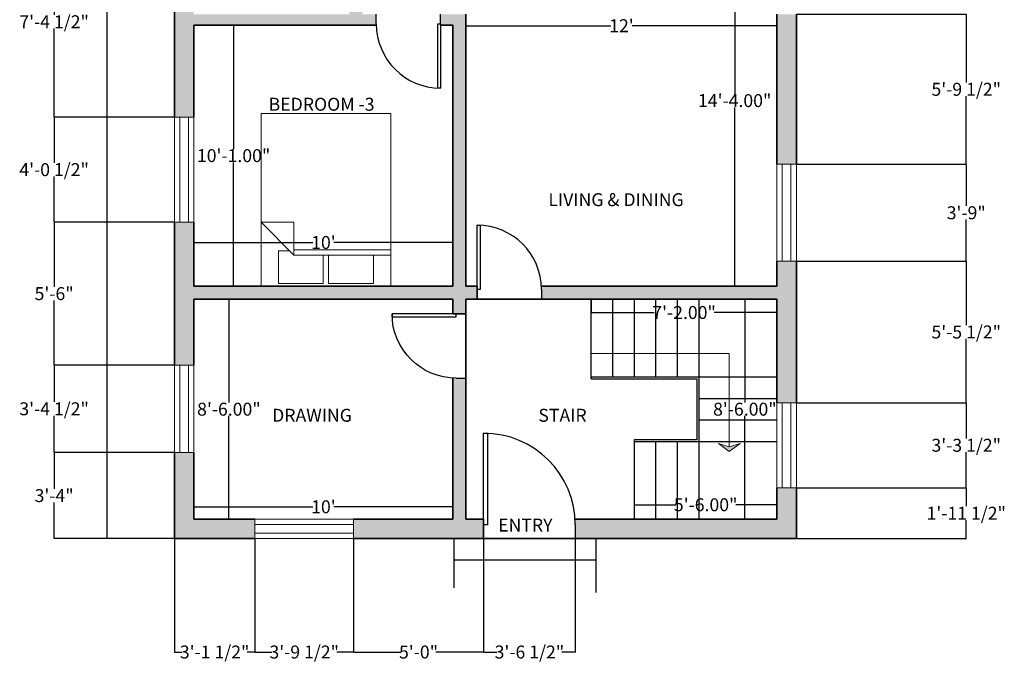
# Model space of a CAD drawing. Units: inches. Extents: x -54 to 402, y -41 to 548.
# Tile 1 of 2: x -54 to 402, y -41 to 261. Entities that reach past the tile are written whole.
import ezdxf

# ---------------------------------------------------------------- set-up
doc = ezdxf.new("R2010")
doc.units = ezdxf.units.IN
doc.header["$MEASUREMENT"] = 0
for name, color, linetype, lineweight in [('A-ANNO-DIMS', 2, 'Continuous', 18), ('A-ANNO-SYMB', 7, 'Continuous', 18), ('A-AREA-IDEN', 7, 'Continuous', 25), ('A-DOOR', 4, 'Continuous', 25), ('A-FLOR-STRS', 7, 'Continuous', 25), ('A-FURN', 8, 'Continuous', 18), ('A-GLAZ', 5, 'Continuous', 18), ('A-WALL', 7, 'Continuous', 35)]:
    doc.layers.add(name, color=color, linetype=linetype, lineweight=lineweight)
doc.layers.add('A-WALL-PATT', color=18, linetype='Continuous', lineweight=13, true_color=0x000000)
doc.styles.get("Standard").update_dxf_attribs({"font": 'arial.ttf'})
doc.dimstyles.get("Standard").update_dxf_attribs({"dimtxt": 6, "dimasz": 0.18, "dimexe": 0.18, "dimexo": 0.0625, "dimgap": 0.09, "dimtad": 0, "dimtih": 1, "dimtoh": 1, "dimzin": 0, "dimdsep": 46, "dimlunit": 3, "dimtxsty": 'Standard', "dimcen": 0.09, "dimadec": 0, "dimazin": 0, "dimtfac": 1, "dimtofl": 0, "dimtmove": 0, "dimatfit": 3, "dimfxl": 1, "dimtolj": 1, "dimtzin": 0, "dimarcsym": 0})

# ---------------------------------------------------------------- blocks, each defined once
blk = doc.blocks.new('*U2')
for p, q in [((0, 0), (0, -6)), ((40, 0), (40, -6))]:
    blk.add_line(p, q)
blk.add_lwpolyline([(0, 0), (0, 40), (1.75, 40), (1.75, 0)], close=True)
blk.add_arc((0, 0), 40, 0, 90)
blk = doc.blocks.new('Bed - Queen')
for p, q in [((0, -80.00003), (0, 0)), ((0, 0), (59.99999, 0)), ((59.99999, 0), (59.99999, -80.00003)), ((7.99999, -1.2), (28.79998, -1.2)), ((7.99999, -14.4), (7.99999, -1.2)), ((28.79998, -1.2), (28.79998, -14.4)), ((31.19999, -1.2), (51.99999, -1.2)), ((31.19999, -14.4), (31.19999, -1.2)), ((51.99999, -1.2), (51.99999, -16.4)), ((0, -14.4), (44.8, -14.4)), ((44.8, -16.8), (0, -16.8)), ((59.99999, -29.6), (44.8, -14.4)), ((44.8, -14.4), (44.8, -29.6)), ((51.99999, -16.4), (46.79936, -16.4)), ((44.8, -29.6), (59.99999, -29.6)), ((59.99999, -80.00003), (0, -80.00003))]:
    blk.add_line(p, q)
blk = doc.blocks.new('*D7')
at = {"layer": 'A-ANNO-DIMS', "color": 0, "lineweight": -2, "transparency": 16777216}
for p, q in [((18.01, 524.86), (-13.3, 524.86)), ((-13.12, 524.68), (-13.12, 275.96)), ((-13.12, 21.04), (-13.12, 269.76)), ((18.01, 20.86), (-13.3, 20.86))]:
    blk.add_line(p, q, dxfattribs=at)
at = {"layer": 'A-ANNO-DIMS', "color": 0, "transparency": 16777216}
for points in [[(-13.15, 524.68), (-13.09, 524.68), (-13.12, 524.86)], [(-13.15, 21.04), (-13.09, 21.04), (-13.12, 20.86)]]:
    blk.add_solid(points, dxfattribs=at)
at = {"layer": 'Defpoints', "color": 0, "transparency": 16777216}
for p in [(18.08, 524.86), (-13.12, 20.86), (18.08, 20.86)]:
    blk.add_point(p, dxfattribs=at)
at = {"layer": 'A-ANNO-DIMS', "color": 0, "transparency": 16777216, "insert": (-13.12, 272.86), "char_height": 6, "attachment_point": 5}
blk.add_mtext("\\A1;42'", dxfattribs=at)
blk = doc.blocks.new('*D8')
at = {"layer": 'A-ANNO-DIMS', "color": 0, "lineweight": -2, "transparency": 16777216}
for p, q in [((211.08, 131.8), (211.08, 125.48)), ((297.08, 131.8), (297.08, 125.48)), ((211.26, 125.66), (240.21, 125.66)), ((296.9, 125.66), (267.94, 125.66))]:
    blk.add_line(p, q, dxfattribs=at)
at = {"layer": 'A-ANNO-DIMS', "color": 0, "transparency": 16777216}
for points in [[(211.26, 125.69), (211.26, 125.63), (211.08, 125.66)], [(296.9, 125.69), (296.9, 125.63), (297.08, 125.66)]]:
    blk.add_solid(points, dxfattribs=at)
at = {"layer": 'Defpoints', "color": 0, "transparency": 16777216}
for p in [(211.08, 131.86), (297.08, 131.86), (297.08, 125.66)]:
    blk.add_point(p, dxfattribs=at)
at = {"layer": 'A-ANNO-DIMS', "color": 0, "transparency": 16777216, "insert": (254.08, 125.66), "char_height": 6, "attachment_point": 5}
blk.add_mtext('\\A1;7\'-2.00"', dxfattribs=at)
blk = doc.blocks.new('*D9')
at = {"layer": 'A-ANNO-DIMS', "color": 0, "lineweight": -2, "transparency": 16777216}
for p, q in [((231.08, 29.92), (231.08, 36.75)), ((231.26, 36.57), (250.19, 36.57)), ((296.9, 36.57), (277.97, 36.57)), ((297.08, 29.92), (297.08, 36.75))]:
    blk.add_line(p, q, dxfattribs=at)
at = {"layer": 'A-ANNO-DIMS', "color": 0, "transparency": 16777216}
for points in [[(231.26, 36.6), (231.26, 36.54), (231.08, 36.57)], [(296.9, 36.6), (296.9, 36.54), (297.08, 36.57)]]:
    blk.add_solid(points, dxfattribs=at)
at = {"layer": 'Defpoints', "color": 0, "transparency": 16777216}
for p in [(297.08, 36.57), (231.08, 29.86), (297.08, 29.86)]:
    blk.add_point(p, dxfattribs=at)
at = {"layer": 'A-ANNO-DIMS', "color": 0, "transparency": 16777216, "insert": (264.08, 36.57), "char_height": 6, "attachment_point": 5}
blk.add_mtext('\\A1;5\'-6.00"', dxfattribs=at)
blk = doc.blocks.new('*D10')
at = {"layer": 'A-ANNO-DIMS', "color": 0, "lineweight": -2, "transparency": 16777216}
for p, q in [((297.01, 131.86), (282.05, 131.86)), ((282.23, 131.68), (282.23, 84.01)), ((282.23, 30.04), (282.23, 77.71)), ((297.01, 29.86), (282.05, 29.86))]:
    blk.add_line(p, q, dxfattribs=at)
at = {"layer": 'A-ANNO-DIMS', "color": 0, "transparency": 16777216}
for points in [[(282.2, 131.68), (282.26, 131.68), (282.23, 131.86)], [(282.2, 30.04), (282.26, 30.04), (282.23, 29.86)]]:
    blk.add_solid(points, dxfattribs=at)
at = {"layer": 'Defpoints', "color": 0, "transparency": 16777216}
for p in [(297.08, 131.86), (282.23, 29.86), (297.08, 29.86)]:
    blk.add_point(p, dxfattribs=at)
at = {"layer": 'A-ANNO-DIMS', "color": 0, "transparency": 16777216, "insert": (282.23, 80.86), "char_height": 6, "attachment_point": 5}
blk.add_mtext('\\A1;8\'-6.00"', dxfattribs=at)
blk = doc.blocks.new('*D11')
at = {"layer": 'A-ANNO-DIMS', "color": 0, "lineweight": -2, "transparency": 16777216}
for p, q in [((27.08, 29.92), (27.08, 35.81)), ((27.26, 35.63), (82.18, 35.63)), ((146.9, 35.63), (91.98, 35.63)), ((147.08, 29.92), (147.08, 35.81))]:
    blk.add_line(p, q, dxfattribs=at)
at = {"layer": 'A-ANNO-DIMS', "color": 0, "transparency": 16777216}
for points in [[(27.26, 35.66), (27.26, 35.6), (27.08, 35.63)], [(146.9, 35.66), (146.9, 35.6), (147.08, 35.63)]]:
    blk.add_solid(points, dxfattribs=at)
at = {"layer": 'Defpoints', "color": 0, "transparency": 16777216}
for p in [(147.08, 35.63), (27.08, 29.86), (147.08, 29.86)]:
    blk.add_point(p, dxfattribs=at)
at = {"layer": 'A-ANNO-DIMS', "color": 0, "transparency": 16777216, "insert": (87.08, 35.63), "char_height": 6, "attachment_point": 5}
blk.add_mtext("\\A1;10'", dxfattribs=at)
blk = doc.blocks.new('*D12')
at = {"layer": 'A-ANNO-DIMS', "color": 0, "lineweight": -2, "transparency": 16777216}
for p, q in [((27.14, 131.86), (43.5, 131.86)), ((43.32, 131.68), (43.32, 84.01)), ((43.32, 30.04), (43.32, 77.71)), ((27.14, 29.86), (43.5, 29.86))]:
    blk.add_line(p, q, dxfattribs=at)
at = {"layer": 'A-ANNO-DIMS', "color": 0, "transparency": 16777216}
for points in [[(43.29, 131.68), (43.35, 131.68), (43.32, 131.86)], [(43.29, 30.04), (43.35, 30.04), (43.32, 29.86)]]:
    blk.add_solid(points, dxfattribs=at)
at = {"layer": 'Defpoints', "color": 0, "transparency": 16777216}
for p in [(27.08, 131.86), (27.08, 29.86), (43.32, 29.86)]:
    blk.add_point(p, dxfattribs=at)
at = {"layer": 'A-ANNO-DIMS', "color": 0, "transparency": 16777216, "insert": (43.32, 80.86), "char_height": 6, "attachment_point": 5}
blk.add_mtext('\\A1;8\'-6.00"', dxfattribs=at)
blk = doc.blocks.new('*D13')
at = {"layer": 'A-ANNO-DIMS', "color": 0, "lineweight": -2, "transparency": 16777216}
for p, q in [((27.08, 137.92), (27.08, 158.29)), ((27.26, 158.11), (82.18, 158.11)), ((146.9, 158.11), (91.98, 158.11)), ((147.08, 137.92), (147.08, 158.29))]:
    blk.add_line(p, q, dxfattribs=at)
at = {"layer": 'A-ANNO-DIMS', "color": 0, "transparency": 16777216}
for points in [[(27.26, 158.14), (27.26, 158.08), (27.08, 158.11)], [(146.9, 158.14), (146.9, 158.08), (147.08, 158.11)]]:
    blk.add_solid(points, dxfattribs=at)
at = {"layer": 'Defpoints', "color": 0, "transparency": 16777216}
for p in [(147.08, 158.11), (27.08, 137.86), (147.08, 137.86)]:
    blk.add_point(p, dxfattribs=at)
at = {"layer": 'A-ANNO-DIMS', "color": 0, "transparency": 16777216, "insert": (87.08, 158.11), "char_height": 6, "attachment_point": 5}
blk.add_mtext("\\A1;10'", dxfattribs=at)
blk = doc.blocks.new('*D14')
at = {"layer": 'A-ANNO-DIMS', "color": 0, "lineweight": -2, "transparency": 16777216}
for p, q in [((27.14, 258.86), (45.68, 258.86)), ((45.5, 258.68), (45.5, 201.51)), ((45.5, 138.04), (45.5, 195.21)), ((27.14, 137.86), (45.68, 137.86))]:
    blk.add_line(p, q, dxfattribs=at)
at = {"layer": 'A-ANNO-DIMS', "color": 0, "transparency": 16777216}
for points in [[(45.47, 258.68), (45.53, 258.68), (45.5, 258.86)], [(45.47, 138.04), (45.53, 138.04), (45.5, 137.86)]]:
    blk.add_solid(points, dxfattribs=at)
at = {"layer": 'Defpoints', "color": 0, "transparency": 16777216}
for p in [(27.08, 258.86), (27.08, 137.86), (45.5, 137.86)]:
    blk.add_point(p, dxfattribs=at)
at = {"layer": 'A-ANNO-DIMS', "color": 0, "transparency": 16777216, "insert": (45.5, 198.36), "char_height": 6, "attachment_point": 5}
blk.add_mtext('\\A1;10\'-1.00"', dxfattribs=at)
blk = doc.blocks.new('*D15')
at = {"layer": 'A-ANNO-DIMS', "color": 0, "lineweight": -2, "transparency": 16777216}
for p, q in [((153.08, 263.8), (153.08, 258.38)), ((297.08, 263.8), (297.08, 258.38)), ((153.26, 258.56), (220.18, 258.56)), ((296.9, 258.56), (229.98, 258.56))]:
    blk.add_line(p, q, dxfattribs=at)
at = {"layer": 'A-ANNO-DIMS', "color": 0, "transparency": 16777216}
for points in [[(153.26, 258.59), (153.26, 258.53), (153.08, 258.56)], [(296.9, 258.59), (296.9, 258.53), (297.08, 258.56)]]:
    blk.add_solid(points, dxfattribs=at)
at = {"layer": 'Defpoints', "color": 0, "transparency": 16777216}
for p in [(153.08, 263.86), (297.08, 263.86), (297.08, 258.56)]:
    blk.add_point(p, dxfattribs=at)
at = {"layer": 'A-ANNO-DIMS', "color": 0, "transparency": 16777216, "insert": (225.08, 258.56), "char_height": 6, "attachment_point": 5}
blk.add_mtext("\\A1;12'", dxfattribs=at)
blk = doc.blocks.new('*D16')
at = {"layer": 'A-ANNO-DIMS', "color": 0, "lineweight": -2, "transparency": 16777216}
for p, q in [((297.01, 309.86), (277.33, 309.86)), ((277.51, 309.68), (277.51, 227.01)), ((277.51, 138.04), (277.51, 220.71)), ((297.01, 137.86), (277.33, 137.86))]:
    blk.add_line(p, q, dxfattribs=at)
at = {"layer": 'A-ANNO-DIMS', "color": 0, "transparency": 16777216}
for points in [[(277.48, 309.68), (277.54, 309.68), (277.51, 309.86)], [(277.48, 138.04), (277.54, 138.04), (277.51, 137.86)]]:
    blk.add_solid(points, dxfattribs=at)
at = {"layer": 'Defpoints', "color": 0, "transparency": 16777216}
for p in [(297.08, 309.86), (277.51, 137.86), (297.08, 137.86)]:
    blk.add_point(p, dxfattribs=at)
at = {"layer": 'A-ANNO-DIMS', "color": 0, "transparency": 16777216, "insert": (277.51, 223.86), "char_height": 6, "attachment_point": 5}
blk.add_mtext('\\A1;14\'-4.00"', dxfattribs=at)
blk = doc.blocks.new('*D32')
at = {"layer": 'A-ANNO-DIMS', "color": 0, "lineweight": -2, "transparency": 16777216}
for p, q in [((18.01, 60.78), (-37.79, 60.78)), ((-37.61, 60.6), (-37.61, 43.98)), ((-37.61, 21.04), (-37.61, 37.67)), ((18.01, 20.86), (-37.79, 20.86))]:
    blk.add_line(p, q, dxfattribs=at)
at = {"layer": 'A-ANNO-DIMS', "color": 0, "transparency": 16777216}
for points in [[(-37.64, 60.6), (-37.58, 60.6), (-37.61, 60.78)], [(-37.64, 21.04), (-37.58, 21.04), (-37.61, 20.86)]]:
    blk.add_solid(points, dxfattribs=at)
at = {"layer": 'Defpoints', "color": 0, "transparency": 16777216}
for p in [(-37.61, 60.78), (18.08, 60.78), (18.08, 20.86)]:
    blk.add_point(p, dxfattribs=at)
at = {"layer": 'A-ANNO-DIMS', "color": 0, "transparency": 16777216, "insert": (-37.61, 40.82), "char_height": 6, "attachment_point": 5}
blk.add_mtext('\\A1;3\'-4"', dxfattribs=at)
blk = doc.blocks.new('*D33')
at = {"layer": 'A-ANNO-DIMS', "color": 0, "lineweight": -2, "transparency": 16777216}
for p, q in [((18.01, 101.29), (-37.79, 101.29)), ((-37.61, 101.11), (-37.61, 84.23)), ((-37.61, 60.96), (-37.61, 77.84)), ((18.01, 60.78), (-37.79, 60.78))]:
    blk.add_line(p, q, dxfattribs=at)
at = {"layer": 'A-ANNO-DIMS', "color": 0, "transparency": 16777216}
for points in [[(-37.64, 101.11), (-37.58, 101.11), (-37.61, 101.29)], [(-37.64, 60.96), (-37.58, 60.96), (-37.61, 60.78)]]:
    blk.add_solid(points, dxfattribs=at)
at = {"layer": 'Defpoints', "color": 0, "transparency": 16777216}
for p in [(-37.61, 101.29), (18.08, 101.29), (18.08, 60.78)]:
    blk.add_point(p, dxfattribs=at)
at = {"layer": 'A-ANNO-DIMS', "color": 0, "transparency": 16777216, "insert": (-37.61, 81.04), "char_height": 6, "attachment_point": 5}
blk.add_mtext('\\A1;3\'-4 1/2"', dxfattribs=at)
blk = doc.blocks.new('*D34')
at = {"layer": 'A-ANNO-DIMS', "color": 0, "lineweight": -2, "transparency": 16777216}
for p, q in [((18.01, 167.53), (-37.79, 167.53)), ((-37.61, 167.35), (-37.61, 137.56)), ((-37.61, 101.47), (-37.61, 131.26)), ((18.01, 101.29), (-37.79, 101.29))]:
    blk.add_line(p, q, dxfattribs=at)
at = {"layer": 'A-ANNO-DIMS', "color": 0, "transparency": 16777216}
for points in [[(-37.64, 167.35), (-37.58, 167.35), (-37.61, 167.53)], [(-37.64, 101.47), (-37.58, 101.47), (-37.61, 101.29)]]:
    blk.add_solid(points, dxfattribs=at)
at = {"layer": 'Defpoints', "color": 0, "transparency": 16777216}
for p in [(-37.61, 167.53), (18.08, 167.53), (18.08, 101.29)]:
    blk.add_point(p, dxfattribs=at)
at = {"layer": 'A-ANNO-DIMS', "color": 0, "transparency": 16777216, "insert": (-37.61, 134.41), "char_height": 6, "attachment_point": 5}
blk.add_mtext('\\A1;5\'-6"', dxfattribs=at)
blk = doc.blocks.new('*D35')
at = {"layer": 'A-ANNO-DIMS', "color": 0, "lineweight": -2, "transparency": 16777216}
for p, q in [((18.01, 216.22), (-37.79, 216.22)), ((-37.61, 216.04), (-37.61, 195.07)), ((-37.61, 167.71), (-37.61, 188.68)), ((18.01, 167.53), (-37.79, 167.53))]:
    blk.add_line(p, q, dxfattribs=at)
at = {"layer": 'A-ANNO-DIMS', "color": 0, "transparency": 16777216}
for points in [[(-37.64, 216.04), (-37.58, 216.04), (-37.61, 216.22)], [(-37.64, 167.71), (-37.58, 167.71), (-37.61, 167.53)]]:
    blk.add_solid(points, dxfattribs=at)
at = {"layer": 'Defpoints', "color": 0, "transparency": 16777216}
for p in [(-37.61, 216.22), (18.08, 216.22), (18.08, 167.53)]:
    blk.add_point(p, dxfattribs=at)
at = {"layer": 'A-ANNO-DIMS', "color": 0, "transparency": 16777216, "insert": (-37.61, 191.87), "char_height": 6, "attachment_point": 5}
blk.add_mtext('\\A1;4\'-0 1/2"', dxfattribs=at)
blk = doc.blocks.new('*D36')
at = {"layer": 'A-ANNO-DIMS', "color": 0, "lineweight": -2, "transparency": 16777216}
for p, q in [((18.01, 304.58), (-37.79, 304.58)), ((-37.61, 304.4), (-37.61, 263.59)), ((-37.61, 216.4), (-37.61, 257.21)), ((18.01, 216.22), (-37.79, 216.22))]:
    blk.add_line(p, q, dxfattribs=at)
at = {"layer": 'A-ANNO-DIMS', "color": 0, "transparency": 16777216}
for points in [[(-37.64, 304.4), (-37.58, 304.4), (-37.61, 304.58)], [(-37.64, 216.4), (-37.58, 216.4), (-37.61, 216.22)]]:
    blk.add_solid(points, dxfattribs=at)
at = {"layer": 'Defpoints', "color": 0, "transparency": 16777216}
for p in [(-37.61, 304.58), (18.08, 304.58), (18.08, 216.22)]:
    blk.add_point(p, dxfattribs=at)
at = {"layer": 'A-ANNO-DIMS', "color": 0, "transparency": 16777216, "insert": (-37.61, 260.4), "char_height": 6, "attachment_point": 5}
blk.add_mtext('\\A1;7\'-4 1/2"', dxfattribs=at)
blk = doc.blocks.new('*D39')
at = {"layer": 'A-ANNO-DIMS', "color": 0, "lineweight": -2, "transparency": 16777216}
for p, q in [((306.14, 44.45), (384.91, 44.45)), ((384.73, 44.27), (384.73, 35.85)), ((384.73, 21.04), (384.73, 29.46)), ((306.14, 20.86), (384.91, 20.86))]:
    blk.add_line(p, q, dxfattribs=at)
at = {"layer": 'A-ANNO-DIMS', "color": 0, "transparency": 16777216}
for points in [[(384.7, 44.27), (384.76, 44.27), (384.73, 44.45)], [(384.7, 21.04), (384.76, 21.04), (384.73, 20.86)]]:
    blk.add_solid(points, dxfattribs=at)
at = {"layer": 'Defpoints', "color": 0, "transparency": 16777216}
for p in [(306.08, 44.45), (384.73, 44.45), (306.08, 20.86)]:
    blk.add_point(p, dxfattribs=at)
at = {"layer": 'A-ANNO-DIMS', "color": 0, "transparency": 16777216, "insert": (384.73, 32.65), "char_height": 6, "attachment_point": 5}
blk.add_mtext('\\A1;1\'-11 1/2"', dxfattribs=at)
blk = doc.blocks.new('*D40')
at = {"layer": 'A-ANNO-DIMS', "color": 0, "lineweight": -2, "transparency": 16777216}
for p, q in [((306.14, 83.84), (384.91, 83.84)), ((384.73, 83.66), (384.73, 67.34)), ((384.73, 44.63), (384.73, 60.95)), ((306.14, 44.45), (384.91, 44.45))]:
    blk.add_line(p, q, dxfattribs=at)
at = {"layer": 'A-ANNO-DIMS', "color": 0, "transparency": 16777216}
for points in [[(384.7, 83.66), (384.76, 83.66), (384.73, 83.84)], [(384.7, 44.63), (384.76, 44.63), (384.73, 44.45)]]:
    blk.add_solid(points, dxfattribs=at)
at = {"layer": 'Defpoints', "color": 0, "transparency": 16777216}
for p in [(306.08, 83.84), (384.73, 83.84), (306.08, 44.45)]:
    blk.add_point(p, dxfattribs=at)
at = {"layer": 'A-ANNO-DIMS', "color": 0, "transparency": 16777216, "insert": (384.73, 64.14), "char_height": 6, "attachment_point": 5}
blk.add_mtext('\\A1;3\'-3 1/2"', dxfattribs=at)
blk = doc.blocks.new('*D41')
at = {"layer": 'A-ANNO-DIMS', "color": 0, "lineweight": -2, "transparency": 16777216}
for p, q in [((306.14, 149.43), (384.91, 149.43)), ((384.73, 149.25), (384.73, 119.83)), ((384.73, 84.02), (384.73, 113.44)), ((306.14, 83.84), (384.91, 83.84))]:
    blk.add_line(p, q, dxfattribs=at)
at = {"layer": 'A-ANNO-DIMS', "color": 0, "transparency": 16777216}
for points in [[(384.7, 149.25), (384.76, 149.25), (384.73, 149.43)], [(384.7, 84.02), (384.76, 84.02), (384.73, 83.84)]]:
    blk.add_solid(points, dxfattribs=at)
at = {"layer": 'Defpoints', "color": 0, "transparency": 16777216}
for p in [(306.08, 149.43), (384.73, 149.43), (306.08, 83.84)]:
    blk.add_point(p, dxfattribs=at)
at = {"layer": 'A-ANNO-DIMS', "color": 0, "transparency": 16777216, "insert": (384.73, 116.63), "char_height": 6, "attachment_point": 5}
blk.add_mtext('\\A1;5\'-5 1/2"', dxfattribs=at)
blk = doc.blocks.new('*D42')
at = {"layer": 'A-ANNO-DIMS', "color": 0, "lineweight": -2, "transparency": 16777216}
for p, q in [((306.14, 194.33), (384.91, 194.33)), ((384.73, 194.15), (384.73, 175.04)), ((384.73, 149.61), (384.73, 168.73)), ((306.14, 149.43), (384.91, 149.43))]:
    blk.add_line(p, q, dxfattribs=at)
at = {"layer": 'A-ANNO-DIMS', "color": 0, "transparency": 16777216}
for points in [[(384.7, 194.15), (384.76, 194.15), (384.73, 194.33)], [(384.7, 149.61), (384.76, 149.61), (384.73, 149.43)]]:
    blk.add_solid(points, dxfattribs=at)
at = {"layer": 'Defpoints', "color": 0, "transparency": 16777216}
for p in [(306.08, 194.33), (384.73, 194.33), (306.08, 149.43)]:
    blk.add_point(p, dxfattribs=at)
at = {"layer": 'A-ANNO-DIMS', "color": 0, "transparency": 16777216, "insert": (384.73, 171.88), "char_height": 6, "attachment_point": 5}
blk.add_mtext('\\A1;3\'-9"', dxfattribs=at)
blk = doc.blocks.new('*D43')
at = {"layer": 'A-ANNO-DIMS', "color": 0, "lineweight": -2, "transparency": 16777216}
for p, q in [((306.14, 263.86), (384.91, 263.86)), ((384.73, 263.68), (384.73, 232.29)), ((384.73, 194.51), (384.73, 225.91)), ((306.14, 194.33), (384.91, 194.33))]:
    blk.add_line(p, q, dxfattribs=at)
at = {"layer": 'A-ANNO-DIMS', "color": 0, "transparency": 16777216}
for points in [[(384.7, 263.68), (384.76, 263.68), (384.73, 263.86)], [(384.7, 194.51), (384.76, 194.51), (384.73, 194.33)]]:
    blk.add_solid(points, dxfattribs=at)
at = {"layer": 'Defpoints', "color": 0, "transparency": 16777216}
for p in [(306.08, 263.86), (384.73, 263.86), (306.08, 194.33)]:
    blk.add_point(p, dxfattribs=at)
at = {"layer": 'A-ANNO-DIMS', "color": 0, "transparency": 16777216, "insert": (384.73, 229.1), "char_height": 6, "attachment_point": 5}
blk.add_mtext('\\A1;5\'-9 1/2"', dxfattribs=at)
blk = doc.blocks.new('*D48')
at = {"layer": 'A-ANNO-DIMS', "color": 0, "lineweight": -2, "transparency": 16777216}
for p, q in [((18.08, 20.8), (18.08, -31.85)), ((55.33, 20.8), (55.33, -31.85)), ((18.26, -31.67), (21.65, -31.67)), ((55.15, -31.67), (51.76, -31.67))]:
    blk.add_line(p, q, dxfattribs=at)
at = {"layer": 'A-ANNO-DIMS', "color": 0, "transparency": 16777216}
for points in [[(18.26, -31.64), (18.26, -31.7), (18.08, -31.67)], [(55.15, -31.64), (55.15, -31.7), (55.33, -31.67)]]:
    blk.add_solid(points, dxfattribs=at)
at = {"layer": 'Defpoints', "color": 0, "transparency": 16777216}
for p in [(18.08, 20.86), (55.33, 20.86), (55.33, -31.67)]:
    blk.add_point(p, dxfattribs=at)
at = {"layer": 'A-ANNO-DIMS', "color": 0, "transparency": 16777216, "insert": (36.71, -31.67), "char_height": 6, "attachment_point": 5}
blk.add_mtext('\\A1;3\'-1 1/2"', dxfattribs=at)
blk = doc.blocks.new('*D49')
at = {"layer": 'A-ANNO-DIMS', "color": 0, "lineweight": -2, "transparency": 16777216}
for p, q in [((55.33, 20.8), (55.33, -31.85)), ((101.04, 20.8), (101.04, -31.85)), ((55.51, -31.67), (63.13, -31.67)), ((100.86, -31.67), (93.24, -31.67))]:
    blk.add_line(p, q, dxfattribs=at)
at = {"layer": 'A-ANNO-DIMS', "color": 0, "transparency": 16777216}
for points in [[(55.51, -31.64), (55.51, -31.7), (55.33, -31.67)], [(100.86, -31.64), (100.86, -31.7), (101.04, -31.67)]]:
    blk.add_solid(points, dxfattribs=at)
at = {"layer": 'Defpoints', "color": 0, "transparency": 16777216}
for p in [(55.33, 20.86), (101.04, 20.86), (101.04, -31.67)]:
    blk.add_point(p, dxfattribs=at)
at = {"layer": 'A-ANNO-DIMS', "color": 0, "transparency": 16777216, "insert": (78.19, -31.67), "char_height": 6, "attachment_point": 5}
blk.add_mtext('\\A1;3\'-9 1/2"', dxfattribs=at)
blk = doc.blocks.new('*D50')
at = {"layer": 'A-ANNO-DIMS', "color": 0, "lineweight": -2, "transparency": 16777216}
for p, q in [((101.04, 20.8), (101.04, -31.85)), ((161.22, 20.8), (161.22, -31.85)), ((101.22, -31.67), (123.07, -31.67)), ((161.04, -31.67), (139.2, -31.67))]:
    blk.add_line(p, q, dxfattribs=at)
at = {"layer": 'A-ANNO-DIMS', "color": 0, "transparency": 16777216}
for points in [[(101.22, -31.64), (101.22, -31.7), (101.04, -31.67)], [(161.04, -31.64), (161.04, -31.7), (161.22, -31.67)]]:
    blk.add_solid(points, dxfattribs=at)
at = {"layer": 'Defpoints', "color": 0, "transparency": 16777216}
for p in [(101.04, 20.86), (161.22, 20.86), (161.22, -31.67)]:
    blk.add_point(p, dxfattribs=at)
at = {"layer": 'A-ANNO-DIMS', "color": 0, "transparency": 16777216, "insert": (131.13, -31.67), "char_height": 6, "attachment_point": 5}
blk.add_mtext('\\A1;5\'-0"', dxfattribs=at)
blk = doc.blocks.new('*D51')
at = {"layer": 'A-ANNO-DIMS', "color": 0, "lineweight": -2, "transparency": 16777216}
for p, q in [((161.22, 20.8), (161.22, -31.85)), ((203.72, 20.8), (203.72, -31.85)), ((161.4, -31.67), (167.42, -31.67)), ((203.54, -31.67), (197.53, -31.67))]:
    blk.add_line(p, q, dxfattribs=at)
at = {"layer": 'A-ANNO-DIMS', "color": 0, "transparency": 16777216}
for points in [[(161.4, -31.64), (161.4, -31.7), (161.22, -31.67)], [(203.54, -31.64), (203.54, -31.7), (203.72, -31.67)]]:
    blk.add_solid(points, dxfattribs=at)
at = {"layer": 'Defpoints', "color": 0, "transparency": 16777216}
for p in [(161.22, 20.86), (203.72, 20.86), (203.72, -31.67)]:
    blk.add_point(p, dxfattribs=at)
at = {"layer": 'A-ANNO-DIMS', "color": 0, "transparency": 16777216, "insert": (182.47, -31.67), "char_height": 6, "attachment_point": 5}
blk.add_mtext('\\A1;3\'-6 1/2"', dxfattribs=at)

msp = doc.modelspace()

# ---------------------------------------------------------------- hatches: boundary and pattern name
at = {"layer": 'A-ANNO-SYMB'}
h = msp.add_hatch(color=256, dxfattribs=at)
h.dxf.hatch_style = 1
h.paths.add_polyline_path([(280.116, 65.005), (274.889, 63.445), (269.955, 65.034), (274.889, 61.274)])
at = {"layer": 'A-WALL-PATT'}
h = msp.add_hatch(color=256, dxfattribs=at)
h.dxf.hatch_style = 1
h.paths.add_polyline_path([(306.077, 149.429), (297.077, 149.429), (297.077, 137.861), (188.036, 137.861, -0.0129064), (188.075, 136.326), (188.075, 131.861), (297.077, 131.861), (297.077, 83.839), (306.077, 83.839)])
h.paths.add_polyline_path([(306.077, 263.861), (297.077, 263.861), (297.077, 194.333), (306.077, 194.333)])
h.paths.add_polyline_path([(306.077, 44.446), (297.077, 44.446), (297.077, 29.861), (203.639, 29.861, -0.015458), (203.72, 27.236), (203.72, 20.861), (306.077, 20.861)])
h.paths.add_polyline_path([(55.334, 29.861), (27.077, 29.861), (27.077, 60.781), (18.077, 60.781), (18.077, 20.861), (55.334, 20.861)])
h.paths.add_polyline_path([(161.225, 27.236), (161.225, 29.861), (153.077, 29.861), (153.077, 95.263), (148.613, 95.263, -0.0129064), (147.077, 95.303), (147.077, 29.861), (101.039, 29.861), (101.039, 20.861), (161.225, 20.861)])
h.paths.add_polyline_path([(158.313, 136.326), (158.313, 137.861), (153.077, 137.861), (153.077, 263.861), (141.33, 263.861), (141.33, 259.397), (141.33, 258.861), (147.077, 258.861), (147.077, 137.861), (27.077, 137.861), (27.077, 167.529), (18.077, 167.529), (18.077, 101.294), (27.077, 101.294), (27.077, 131.861), (147.077, 131.861), (147.077, 125.025), (148.613, 125.025), (153.077, 125.025), (153.077, 131.861), (158.313, 131.861)])
h.paths.add_polyline_path([(111.568, 263.861), (105.077, 263.861), (105.077, 293.745), (99.077, 293.745), (99.077, 263.861), (27.077, 263.861), (27.077, 304.579), (18.077, 304.579), (18.077, 216.221), (27.077, 216.221), (27.077, 258.861), (111.573, 258.861, -0.0045002), (111.568, 259.397)])
h.paths.add_polyline_path([(112.102, 364.326, -0.0129064), (112.142, 365.861), (27.077, 365.861), (27.077, 402.028), (18.077, 402.028), (18.077, 335.061), (27.077, 335.061), (27.077, 359.861), (99.077, 359.861), (99.077, 331.859), (105.077, 331.859), (105.077, 359.861), (112.102, 359.861)])

# ---------------------------------------------------------------- linework, layer by layer
at = {"layer": 'A-ANNO-SYMB'}
for p, q in [((211.077, 106.597), (274.889, 106.597)), ((274.889, 106.597), (274.889, 63.445)), ((274.889, 61.274), (269.955, 65.034)), ((274.889, 63.445), (269.955, 65.034)), ((274.889, 61.274), (280.116, 65.005)), ((280.116, 65.005), (274.889, 61.274)), ((274.889, 63.445), (280.116, 65.005))]:
    msp.add_line(p, q, dxfattribs=at)
at = {"layer": 'A-DOOR'}
msp.add_lwpolyline([(161.225, 27.361), (163.084, 27.361)], dxfattribs=at)
at = {"layer": 'A-FLOR-STRS'}
for p, q in [((261.077, 95.861), (297.077, 95.861)), ((261.077, 85.861), (297.077, 85.861)), ((261.077, 75.861), (297.077, 75.861)), ((261.077, 65.861), (297.077, 65.861)), ((147.465, 20.861), (147.465, -1.916)), ((213.19, 20.861), (213.19, -4.018)), ((147.465, 11.118), (213.19, 11.118))]:
    msp.add_line(p, q, dxfattribs=at)
for points in [[(211.077, 94.861), (211.077, 131.861)], [(221.077, 95.861), (221.077, 131.861)], [(231.077, 95.861), (231.077, 131.861)], [(241.077, 95.861), (241.077, 131.861)], [(251.077, 95.861), (251.077, 131.861)], [(261.077, 29.861), (261.077, 131.861)], [(211.077, 95.861), (261.077, 95.861)], [(211.077, 94.861), (260.077, 94.861)], [(260.077, 66.861), (260.077, 94.861)], [(231.077, 29.861), (231.077, 66.861)], [(231.077, 66.861), (260.077, 66.861)], [(231.077, 65.861), (261.077, 65.861)], [(241.077, 29.861), (241.077, 65.861)], [(251.077, 29.861), (251.077, 65.861)]]:
    msp.add_lwpolyline(points, dxfattribs=at)
at = {"layer": 'A-GLAZ'}
for p, q in [((27.077, 216.221), (18.077, 216.221)), ((297.077, 194.333), (306.077, 194.333)), ((27.077, 167.529), (18.077, 167.529)), ((297.077, 149.429), (306.077, 149.429)), ((27.077, 101.294), (18.077, 101.294)), ((297.077, 83.839), (306.077, 83.839)), ((27.077, 60.781), (18.077, 60.781)), ((297.077, 44.446), (306.077, 44.446)), ((55.334, 29.861), (55.334, 20.861)), ((101.039, 29.861), (101.039, 20.861))]:
    msp.add_line(p, q, dxfattribs=at)
for points in [[(18.077, 216.221), (27.077, 216.221), (27.077, 167.529), (18.077, 167.529)], [(297.077, 194.333), (306.077, 194.333), (306.077, 149.429), (297.077, 149.429)], [(18.077, 101.294), (27.077, 101.294), (27.077, 60.781), (18.077, 60.781)], [(297.077, 83.839), (306.077, 83.839), (306.077, 44.446), (297.077, 44.446)], [(55.334, 29.861), (101.039, 29.861), (101.039, 20.861), (55.334, 20.861)]]:
    msp.add_lwpolyline(points, close=True, dxfattribs=at)
for points in [[(20.577, 216.221), (20.577, 167.529)], [(24.577, 216.221), (24.577, 167.529)], [(299.577, 149.429), (299.577, 194.333)], [(303.577, 149.429), (303.577, 194.333)], [(20.577, 101.294), (20.577, 60.781)], [(24.577, 101.294), (24.577, 60.781)], [(299.577, 44.446), (299.577, 83.839)], [(303.577, 44.446), (303.577, 83.839)], [(55.334, 27.361), (101.039, 27.361)], [(55.334, 23.361), (101.039, 23.361)]]:
    msp.add_lwpolyline(points, dxfattribs=at)
at = {"layer": 'A-WALL'}
for p, q in [((297.077, 137.861), (297.077, 149.429)), ((158.313, 137.861), (158.313, 131.861)), ((147.077, 125.025), (153.077, 125.025)), ((161.225, 29.861), (161.225, 20.861))]:
    msp.add_line(p, q, dxfattribs=at)
for points in [[(18.077, 304.579), (18.077, 216.221)], [(153.077, 137.861), (153.077, 263.861)], [(297.077, 194.333), (297.077, 263.861)], [(306.077, 194.333), (306.077, 263.861)], [(27.077, 258.861), (27.077, 216.221)], [(111.573, 258.861), (27.077, 258.861)], [(147.077, 258.861), (141.33, 258.861)], [(147.077, 258.861), (147.077, 137.861)], [(18.077, 167.529), (18.077, 101.294)], [(27.077, 167.529), (27.077, 137.861)], [(297.077, 137.861), (297.077, 149.429)], [(306.077, 83.839), (306.077, 149.429)], [(27.077, 137.861), (147.077, 137.861)], [(153.077, 137.861), (158.313, 137.861)], [(188.036, 137.861), (297.077, 137.861)], [(27.077, 131.861), (147.077, 131.861)], [(27.077, 131.861), (27.077, 101.294)], [(147.077, 131.861), (147.077, 125.025)], [(153.077, 29.861), (153.077, 131.861)], [(153.077, 131.861), (297.077, 131.861)], [(297.077, 83.839), (297.077, 131.861)], [(147.077, 95.303), (147.077, 29.861)], [(18.077, 60.781), (18.077, 20.861), (55.334, 20.861)], [(27.077, 60.781), (27.077, 29.861)], [(101.039, 20.861), (306.077, 20.861), (306.077, 44.446)], [(297.077, 29.861), (297.077, 44.446)], [(27.077, 29.861), (55.334, 29.861)], [(101.039, 29.861), (147.077, 29.861)], [(153.077, 29.861), (161.225, 29.861)], [(203.639, 29.861), (297.077, 29.861)]]:
    msp.add_lwpolyline(points, dxfattribs=at)

# ---------------------------------------------------------------- block references
at = {"layer": 'A-DOOR', "yscale": 0.7440482998037414, "zscale": 0.7440482998037414}
for p, xscale, rotation in [((141.33, 259.397), 0.7440482998037414, 180), ((148.613, 125.025), -0.7440482998037414, 90)]:
    msp.add_blockref('*U2', p, dxfattribs=dict(at, xscale=xscale, rotation=rotation))
at = {"layer": 'A-DOOR'}
for p, xscale, yscale, zscale in [((158.313, 136.326), 0.7440482998037414, 0.7440482998037414, 0.7440482998037414), ((161.225, 27.236), 1.06238410725418, 1.06238410725418, 1.06238410725418)]:
    msp.add_blockref('*U2', p, dxfattribs=dict(at, xscale=xscale, yscale=yscale, zscale=zscale))
at = {"layer": 'A-FURN', "rotation": 180}
msp.add_blockref('Bed - Queen', (118.229, 137.861), dxfattribs=at)

# ---------------------------------------------------------------- texts
at = {"layer": 'A-AREA-IDEN', "char_height": 6, "attachment_point": 1}
for s, insert in [('BEDROOM -3', (61.717, 225.168)), ('LIVING & DINING', (191.262, 180.948)), ('DRAWING', (63.327, 81.039)), ('STAIR', (186.604, 81.039)), ('ENTRY', (167.973, 30.154))]:
    msp.add_mtext_dynamic_manual_height_columns(s, width=186.62834, gutter_width=1, heights=[0], dxfattribs=dict(at, insert=insert))

# ---------------------------------------------------------------- dimensions: what is measured, and where the dimension line sits
at = {"layer": 'A-ANNO-DIMS'}
for base, p1, p2, override, picture, middle in [((-13.116, 20.861), (18.077, 524.861), (18.077, 20.861), {"dimclrd": 0, "dimclre": 0, "dimclrt": 0}, '*D7', (-13.116, 272.861)), ((277.507, 137.861), (297.077, 309.861), (297.077, 137.861), {"dimclrd": 0, "dimclre": 0, "dimclrt": 0}, '*D16', (277.507, 223.861)), ((-37.609, 304.579), (18.077, 216.221), (18.077, 304.579), {"dimdec": 1, "dimlfac": 1, "dimrnd": 0, "dimzin": 1, "dimdsep": 46, "dimlunit": 4, "dimfrac": 2}, '*D36', (-37.609, 260.4)), ((384.727, 263.861), (306.077, 194.333), (306.077, 263.861), {"dimdec": 1, "dimlfac": 1, "dimrnd": 0, "dimzin": 1, "dimdsep": 46, "dimlunit": 4, "dimfrac": 2}, '*D43', (384.727, 229.097)), ((45.497, 137.861), (27.077, 258.861), (27.077, 137.861), {"dimclrd": 0, "dimclre": 0, "dimclrt": 0}, '*D14', (45.497, 198.361)), ((-37.609, 216.221), (18.077, 167.529), (18.077, 216.221), {"dimdec": 1, "dimlfac": 1, "dimrnd": 0, "dimzin": 1, "dimdsep": 46, "dimlunit": 4, "dimfrac": 2}, '*D35', (-37.609, 191.875)), ((384.727, 194.333), (306.077, 149.429), (306.077, 194.333), {"dimdec": 1, "dimlfac": 1, "dimrnd": 0, "dimzin": 1, "dimdsep": 46, "dimlunit": 4, "dimfrac": 2}, '*D42', (384.727, 171.881)), ((-37.609, 167.529), (18.077, 101.294), (18.077, 167.529), {"dimdec": 1, "dimlfac": 1, "dimrnd": 0, "dimzin": 1, "dimdsep": 46, "dimlunit": 4, "dimfrac": 2}, '*D34', (-37.609, 134.412)), ((384.727, 149.429), (306.077, 83.839), (306.077, 149.429), {"dimdec": 1, "dimlfac": 1, "dimrnd": 0, "dimzin": 1, "dimdsep": 46, "dimlunit": 4, "dimfrac": 2}, '*D41', (384.727, 116.634)), ((43.322, 29.861), (27.077, 131.861), (27.077, 29.861), {"dimclrd": 0, "dimclre": 0, "dimclrt": 0}, '*D12', (43.322, 80.861)), ((282.233, 29.861), (297.077, 131.861), (297.077, 29.861), {"dimclrd": 0, "dimclre": 0, "dimclrt": 0}, '*D10', (282.233, 80.861)), ((-37.609, 101.294), (18.077, 60.781), (18.077, 101.294), {"dimdec": 1, "dimlfac": 1, "dimrnd": 0, "dimzin": 1, "dimdsep": 46, "dimlunit": 4, "dimfrac": 2}, '*D33', (-37.609, 81.038)), ((384.727, 83.839), (306.077, 44.446), (306.077, 83.839), {"dimdec": 1, "dimlfac": 1, "dimrnd": 0, "dimzin": 1, "dimdsep": 46, "dimlunit": 4, "dimfrac": 2}, '*D40', (384.727, 64.142)), ((-37.609, 60.781), (18.077, 20.861), (18.077, 60.781), {"dimdec": 1, "dimlfac": 1, "dimrnd": 0, "dimzin": 1, "dimdsep": 46, "dimlunit": 4, "dimfrac": 2}, '*D32', (-37.609, 40.821)), ((384.727, 44.446), (306.077, 20.861), (306.077, 44.446), {"dimdec": 1, "dimlfac": 1, "dimrnd": 0, "dimzin": 1, "dimdsep": 46, "dimlunit": 4, "dimfrac": 2}, '*D39', (384.727, 32.654))]:
    dim = msp.add_linear_dim(base=base, p1=p1, p2=p2, angle=90, dimstyle='Standard', override=override, dxfattribs=at)
    dim.commit()
    dim.dimension.update_dxf_attribs({"geometry": picture, "text_midpoint": middle})
for base, p1, p2, override, picture, middle in [((297.077, 258.564), (153.077, 263.861), (297.077, 263.861), {"dimclrd": 0, "dimclre": 0, "dimclrt": 0}, '*D15', (225.077, 258.564)), ((147.077, 158.105), (27.077, 137.861), (147.077, 137.861), {"dimclrd": 0, "dimclre": 0, "dimclrt": 0}, '*D13', (87.077, 158.105)), ((297.077, 125.658), (211.077, 131.861), (297.077, 131.861), {"dimclrd": 0, "dimclre": 0, "dimclrt": 0}, '*D8', (254.077, 125.658)), ((147.077, 35.634), (27.077, 29.861), (147.077, 29.861), {"dimclrd": 0, "dimclre": 0, "dimclrt": 0}, '*D11', (87.077, 35.634)), ((297.077, 36.572), (231.077, 29.861), (297.077, 29.861), {"dimclrd": 0, "dimclre": 0, "dimclrt": 0}, '*D9', (264.077, 36.572)), ((55.334, -31.668), (18.077, 20.861), (55.334, 20.861), {"dimdec": 1, "dimlfac": 1, "dimrnd": 0, "dimzin": 1, "dimdsep": 46, "dimlunit": 4, "dimfrac": 2}, '*D48', (36.705, -31.668)), ((101.039, -31.668), (55.334, 20.861), (101.039, 20.861), {"dimdec": 1, "dimlfac": 1, "dimrnd": 0, "dimzin": 1, "dimdsep": 46, "dimlunit": 4, "dimfrac": 2}, '*D49', (78.186, -31.668)), ((161.225, -31.668), (101.039, 20.861), (161.225, 20.861), {"dimdec": 1, "dimlfac": 1, "dimrnd": 0, "dimzin": 1, "dimdsep": 46, "dimlunit": 4, "dimfrac": 2}, '*D50', (131.132, -31.668)), ((203.72, -31.668), (161.225, 20.861), (203.72, 20.861), {"dimdec": 1, "dimlfac": 1, "dimrnd": 0, "dimzin": 1, "dimdsep": 46, "dimlunit": 4, "dimfrac": 2}, '*D51', (182.472, -31.668))]:
    dim = msp.add_linear_dim(base=base, p1=p1, p2=p2, dimstyle='Standard', override=override, dxfattribs=at)
    dim.commit()
    dim.dimension.update_dxf_attribs({"geometry": picture, "text_midpoint": middle})

doc.saveas('drawing.dxf')
